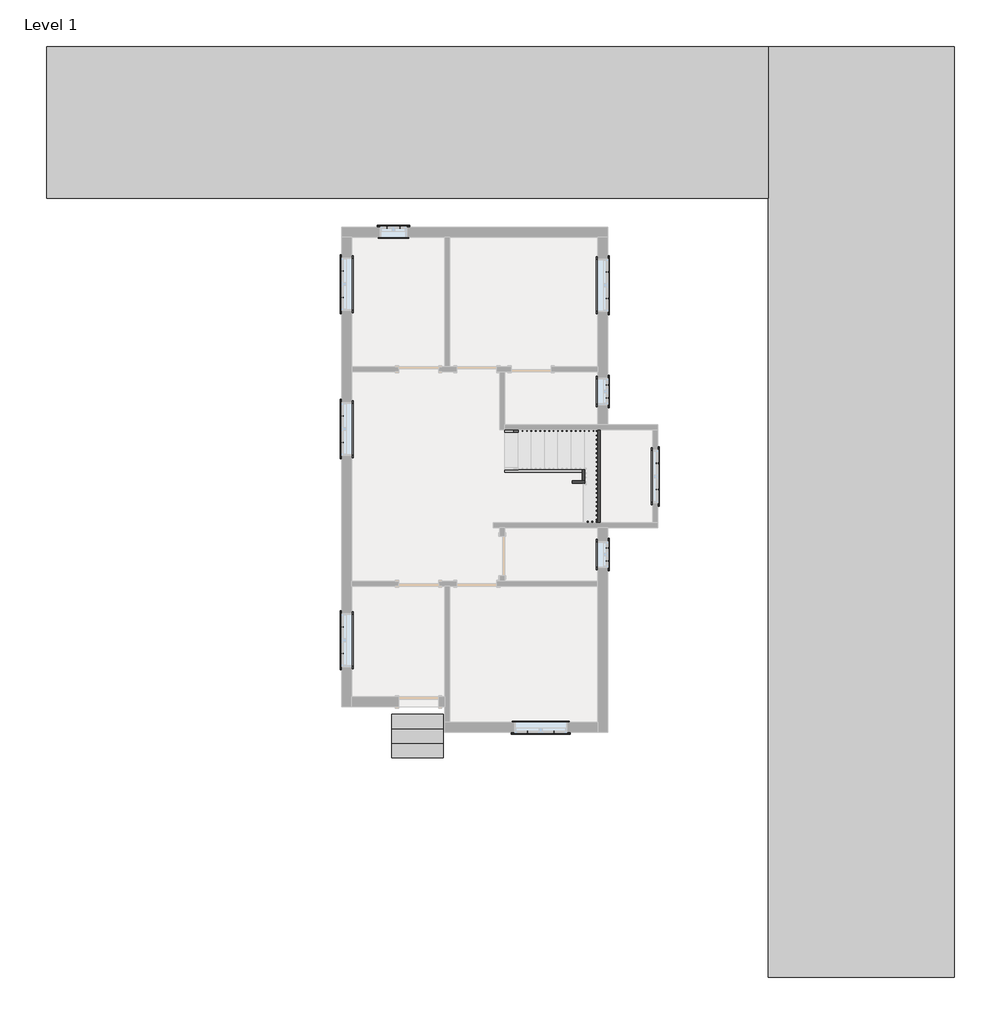
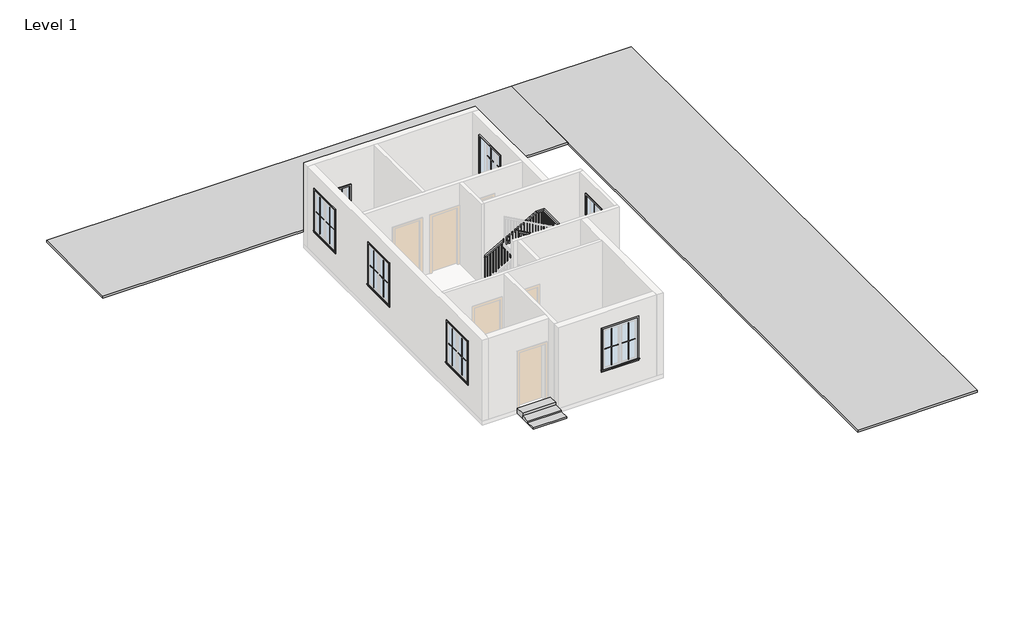
# One storey, part 2 of 2: 38 proxies, 4 members, 1 railing.
"""IFC4 building model written with IfcOpenShell, lengths in millimetres."""

from ifc_helpers import new_model, si_unit, frame, origin, place, context, project, spatial, polyline, outline, extrude, faceted_brep, transform, mapped, element, save
from components import generic_models_1_generic_models_1_85262742, generic_models_2_generic_models_2_51d3bdcd, muntin_pattern_2x2_muntin_pattern_2x2_6dad3731, muntin_pattern_2x2_muntin_pattern_2x2_a30a3345, muntin_pattern_2x2_muntin_pattern_2x2_53152e2c, muntin_pattern_2x2_muntin_pattern_2x2_e8f3e573, trim_window_exterior_flat_with_sill_92b9b949, trim_window_exterior_flat_with_sill_a665a915, trim_window_interior_flat_picture_frame_3bb882cf, trim_window_interior_flat_picture_frame_d485c387

model = new_model("IFC4")

# Units and contexts
model_context = context("Model", 3, world=origin())
ifc_project = project(units=[si_unit("LENGTHUNIT", "METRE", prefix="MILLI")], contexts=[model_context])

# Site, building, storey
site = spatial("IfcSite", under=ifc_project)
building = spatial("IfcBuilding", under=site)
storey = spatial("IfcBuildingStorey", under=building, Name="Level 1", Elevation=0.0)

# Proxies
placement = place(None, origin())
generic_models_1_generic_models_1_shape = generic_models_1_generic_models_1_85262742(model_context)
element("IfcBuildingElementProxy", 1, Name="Generic Models 1 : Generic Models 1", ObjectType="Generic Models 1 : Generic Models 1", at=placement, inside=storey, context=model_context, shape_type="MappedRepresentation", body=[
    mapped(generic_models_1_generic_models_1_shape, transform((0.0, 0.0, 0.0), x_axis=(1.0, 0.0, 0.0), y_axis=(0.0, 1.0, 0.0), z_axis=(0.0, 0.0, 1.0))),
])
generic_models_2_generic_models_2_shape = generic_models_2_generic_models_2_51d3bdcd(model_context)
element("IfcBuildingElementProxy", 2, Name="Generic Models 2 : Generic Models 2", ObjectType="Generic Models 2 : Generic Models 2", at=placement, inside=storey, context=model_context, shape_type="MappedRepresentation", body=[
    mapped(generic_models_2_generic_models_2_shape, transform((0.0, 0.0, 0.0), x_axis=(1.0, 0.0, 0.0), y_axis=(0.0, 1.0, 0.0), z_axis=(0.0, 0.0, 1.0))),
])
muntin_pattern_2x2_muntin_pattern_2x2_shape = muntin_pattern_2x2_muntin_pattern_2x2_6dad3731(model_context)
element("IfcBuildingElementProxy", 3, Name="Muntin Pattern_2x2 : Muntin Pattern_2x2", ObjectType="Muntin Pattern_2x2 : Muntin Pattern_2x2", at=placement, inside=storey, context=model_context, shape_type="MappedRepresentation", body=[
    mapped(muntin_pattern_2x2_muntin_pattern_2x2_shape, transform((1279.525, 12612.6875, 984.25), x_axis=(0.0, 1.0, 0.0), y_axis=(-1.0, 0.0, 0.0), z_axis=(0.0, 0.0, 1.0))),
])
element("IfcBuildingElementProxy", 4, Name="Muntin Pattern_2x2 : Muntin Pattern_2x2", ObjectType="Muntin Pattern_2x2 : Muntin Pattern_2x2", at=placement, inside=storey, context=model_context, shape_type="MappedRepresentation", body=[
    mapped(muntin_pattern_2x2_muntin_pattern_2x2_shape, transform((7356.475, 13193.7125, 984.25), x_axis=(0.0, -1.0, 0.0), y_axis=(1.0, 0.0, 0.0), z_axis=(0.0, 0.0, 1.0))),
])
element("IfcBuildingElementProxy", 5, Name="Muntin Pattern_2x2 : Muntin Pattern_2x2", ObjectType="Muntin Pattern_2x2 : Muntin Pattern_2x2", at=placement, inside=storey, context=model_context, shape_type="MappedRepresentation", body=[
    mapped(muntin_pattern_2x2_muntin_pattern_2x2_shape, transform((8499.475, 8812.2125, 984.25), x_axis=(0.0, -1.0, 0.0), y_axis=(1.0, 0.0, 0.0), z_axis=(0.0, 0.0, 1.0))),
])
element("IfcBuildingElementProxy", 6, Name="Muntin Pattern_2x2 : Muntin Pattern_2x2", ObjectType="Muntin Pattern_2x2 : Muntin Pattern_2x2", at=placement, inside=storey, context=model_context, shape_type="MappedRepresentation", body=[
    mapped(muntin_pattern_2x2_muntin_pattern_2x2_shape, transform((6132.5125, 2651.125, 984.25), x_axis=(-1.0, 0.0, 0.0), y_axis=(0.0, -1.0, 0.0), z_axis=(0.0, 0.0, 1.0))),
])
element("IfcBuildingElementProxy", 7, Name="Muntin Pattern_2x2 : Muntin Pattern_2x2", ObjectType="Muntin Pattern_2x2 : Muntin Pattern_2x2", at=placement, inside=storey, context=model_context, shape_type="MappedRepresentation", body=[
    mapped(muntin_pattern_2x2_muntin_pattern_2x2_shape, transform((1279.525, 4452.9375, 984.25), x_axis=(0.0, 1.0, 0.0), y_axis=(-1.0, 0.0, 0.0), z_axis=(0.0, 0.0, 1.0))),
])
element("IfcBuildingElementProxy", 8, Name="Muntin Pattern_2x2 : Muntin Pattern_2x2", ObjectType="Muntin Pattern_2x2 : Muntin Pattern_2x2", at=placement, inside=storey, context=model_context, shape_type="MappedRepresentation", body=[
    mapped(muntin_pattern_2x2_muntin_pattern_2x2_shape, transform((1279.525, 9291.6375, 984.25), x_axis=(0.0, 1.0, 0.0), y_axis=(-1.0, 0.0, 0.0), z_axis=(0.0, 0.0, 1.0))),
])
muntin_pattern_2x2_muntin_pattern_2x2_2_shape = muntin_pattern_2x2_muntin_pattern_2x2_a30a3345(model_context)
element("IfcBuildingElementProxy", 9, Name="Muntin Pattern_2x2 : Muntin Pattern_2x2", ObjectType="Muntin Pattern_2x2 : Muntin Pattern_2x2", at=placement, inside=storey, context=model_context, shape_type="MappedRepresentation", body=[
    mapped(muntin_pattern_2x2_muntin_pattern_2x2_2_shape, transform((1279.525, 13219.1125, 984.25), x_axis=(0.0, -1.0, 0.0), y_axis=(1.0, 0.0, 0.0), z_axis=(0.0, 0.0, 1.0))),
])
element("IfcBuildingElementProxy", 10, Name="Muntin Pattern_2x2 : Muntin Pattern_2x2", ObjectType="Muntin Pattern_2x2 : Muntin Pattern_2x2", at=placement, inside=storey, context=model_context, shape_type="MappedRepresentation", body=[
    mapped(muntin_pattern_2x2_muntin_pattern_2x2_2_shape, transform((7356.475, 12587.2875, 984.25), x_axis=(0.0, 1.0, 0.0), y_axis=(-1.0, 0.0, 0.0), z_axis=(0.0, 0.0, 1.0))),
])
element("IfcBuildingElementProxy", 11, Name="Muntin Pattern_2x2 : Muntin Pattern_2x2", ObjectType="Muntin Pattern_2x2 : Muntin Pattern_2x2", at=placement, inside=storey, context=model_context, shape_type="MappedRepresentation", body=[
    mapped(muntin_pattern_2x2_muntin_pattern_2x2_2_shape, transform((8499.475, 8205.7875, 984.25), x_axis=(0.0, 1.0, 0.0), y_axis=(-1.0, 0.0, 0.0), z_axis=(0.0, 0.0, 1.0))),
])
element("IfcBuildingElementProxy", 12, Name="Muntin Pattern_2x2 : Muntin Pattern_2x2", ObjectType="Muntin Pattern_2x2 : Muntin Pattern_2x2", at=placement, inside=storey, context=model_context, shape_type="MappedRepresentation", body=[
    mapped(muntin_pattern_2x2_muntin_pattern_2x2_2_shape, transform((5526.0875, 2651.125, 984.25), x_axis=(1.0, 0.0, 0.0), y_axis=(0.0, 1.0, 0.0), z_axis=(0.0, 0.0, 1.0))),
])
element("IfcBuildingElementProxy", 13, Name="Muntin Pattern_2x2 : Muntin Pattern_2x2", ObjectType="Muntin Pattern_2x2 : Muntin Pattern_2x2", at=placement, inside=storey, context=model_context, shape_type="MappedRepresentation", body=[
    mapped(muntin_pattern_2x2_muntin_pattern_2x2_2_shape, transform((1279.525, 5059.3625, 984.25), x_axis=(0.0, -1.0, 0.0), y_axis=(1.0, 0.0, 0.0), z_axis=(0.0, 0.0, 1.0))),
])
element("IfcBuildingElementProxy", 14, Name="Muntin Pattern_2x2 : Muntin Pattern_2x2", ObjectType="Muntin Pattern_2x2 : Muntin Pattern_2x2", at=placement, inside=storey, context=model_context, shape_type="MappedRepresentation", body=[
    mapped(muntin_pattern_2x2_muntin_pattern_2x2_2_shape, transform((1279.525, 9898.0625, 984.25), x_axis=(0.0, -1.0, 0.0), y_axis=(1.0, 0.0, 0.0), z_axis=(0.0, 0.0, 1.0))),
])
muntin_pattern_2x2_muntin_pattern_2x2_3_shape = muntin_pattern_2x2_muntin_pattern_2x2_53152e2c(model_context)
element("IfcBuildingElementProxy", 15, Name="Muntin Pattern_2x2 : Muntin Pattern_2x2", ObjectType="Muntin Pattern_2x2 : Muntin Pattern_2x2", at=placement, inside=storey, context=model_context, shape_type="MappedRepresentation", body=[
    mapped(muntin_pattern_2x2_muntin_pattern_2x2_3_shape, transform((2300.2875, 14214.475, 984.25), x_axis=(1.0, 0.0, 0.0), y_axis=(0.0, 1.0, 0.0), z_axis=(0.0, 0.0, 1.0))),
])
element("IfcBuildingElementProxy", 16, Name="Muntin Pattern_2x2 : Muntin Pattern_2x2", ObjectType="Muntin Pattern_2x2 : Muntin Pattern_2x2", at=placement, inside=storey, context=model_context, shape_type="MappedRepresentation", body=[
    mapped(muntin_pattern_2x2_muntin_pattern_2x2_3_shape, transform((7356.475, 10609.2625, 984.25), x_axis=(0.0, -1.0, 0.0), y_axis=(1.0, 0.0, 0.0), z_axis=(0.0, 0.0, 1.0))),
])
element("IfcBuildingElementProxy", 17, Name="Muntin Pattern_2x2 : Muntin Pattern_2x2", ObjectType="Muntin Pattern_2x2 : Muntin Pattern_2x2", at=placement, inside=storey, context=model_context, shape_type="MappedRepresentation", body=[
    mapped(muntin_pattern_2x2_muntin_pattern_2x2_3_shape, transform((7356.475, 6869.1125, 984.25), x_axis=(0.0, -1.0, 0.0), y_axis=(1.0, 0.0, 0.0), z_axis=(0.0, 0.0, 1.0))),
])
muntin_pattern_2x2_muntin_pattern_2x2_4_shape = muntin_pattern_2x2_muntin_pattern_2x2_e8f3e573(model_context)
element("IfcBuildingElementProxy", 18, Name="Muntin Pattern_2x2 : Muntin Pattern_2x2", ObjectType="Muntin Pattern_2x2 : Muntin Pattern_2x2", at=placement, inside=storey, context=model_context, shape_type="MappedRepresentation", body=[
    mapped(muntin_pattern_2x2_muntin_pattern_2x2_4_shape, transform((2601.9125, 14214.475, 984.25), x_axis=(-1.0, 0.0, 0.0), y_axis=(0.0, -1.0, 0.0), z_axis=(0.0, 0.0, 1.0))),
])
element("IfcBuildingElementProxy", 19, Name="Muntin Pattern_2x2 : Muntin Pattern_2x2", ObjectType="Muntin Pattern_2x2 : Muntin Pattern_2x2", at=placement, inside=storey, context=model_context, shape_type="MappedRepresentation", body=[
    mapped(muntin_pattern_2x2_muntin_pattern_2x2_4_shape, transform((7356.475, 10307.6375, 984.25), x_axis=(0.0, 1.0, 0.0), y_axis=(-1.0, 0.0, 0.0), z_axis=(0.0, 0.0, 1.0))),
])
element("IfcBuildingElementProxy", 20, Name="Muntin Pattern_2x2 : Muntin Pattern_2x2", ObjectType="Muntin Pattern_2x2 : Muntin Pattern_2x2", at=placement, inside=storey, context=model_context, shape_type="MappedRepresentation", body=[
    mapped(muntin_pattern_2x2_muntin_pattern_2x2_4_shape, transform((7356.475, 6567.4875, 984.25), x_axis=(0.0, 1.0, 0.0), y_axis=(-1.0, 0.0, 0.0), z_axis=(0.0, 0.0, 1.0))),
])
trim_window_exterior_flat_with_sill_shape = trim_window_exterior_flat_with_sill_92b9b949(model_context)
element("IfcBuildingElementProxy", 21, Name="Trim-Window-Exterior-Flat : with Sill", ObjectType="Trim-Window-Exterior-Flat : with Sill", at=placement, inside=storey, context=model_context, shape_type="MappedRepresentation", body=[
    mapped(trim_window_exterior_flat_with_sill_shape, transform((1270.0, 12915.9, 2438.4), x_axis=(0.0, -1.0, 0.0), y_axis=(0.0, 0.0, 1.0), z_axis=(-1.0, 0.0, 0.0))),
])
element("IfcBuildingElementProxy", 22, Name="Trim-Window-Exterior-Flat : with Sill", ObjectType="Trim-Window-Exterior-Flat : with Sill", at=placement, inside=storey, context=model_context, shape_type="MappedRepresentation", body=[
    mapped(trim_window_exterior_flat_with_sill_shape, transform((7366.0, 12890.5, 2438.4), x_axis=(0.0, 1.0, 0.0), y_axis=(0.0, 0.0, 1.0), z_axis=(1.0, 0.0, 0.0))),
])
element("IfcBuildingElementProxy", 23, Name="Trim-Window-Exterior-Flat : with Sill", ObjectType="Trim-Window-Exterior-Flat : with Sill", at=placement, inside=storey, context=model_context, shape_type="MappedRepresentation", body=[
    mapped(trim_window_exterior_flat_with_sill_shape, transform((8509.0, 8509.0, 2438.4), x_axis=(0.0, 1.0, 0.0), y_axis=(0.0, 0.0, 1.0), z_axis=(1.0, 0.0, 0.0))),
])
element("IfcBuildingElementProxy", 24, Name="Trim-Window-Exterior-Flat : with Sill", ObjectType="Trim-Window-Exterior-Flat : with Sill", at=placement, inside=storey, context=model_context, shape_type="MappedRepresentation", body=[
    mapped(trim_window_exterior_flat_with_sill_shape, transform((5829.3, 2641.6, 2438.4), x_axis=(1.0, 0.0, 0.0), y_axis=(0.0, 0.0, 1.0), z_axis=(0.0, -1.0, 0.0))),
])
element("IfcBuildingElementProxy", 25, Name="Trim-Window-Exterior-Flat : with Sill", ObjectType="Trim-Window-Exterior-Flat : with Sill", at=placement, inside=storey, context=model_context, shape_type="MappedRepresentation", body=[
    mapped(trim_window_exterior_flat_with_sill_shape, transform((1270.0, 4756.15, 2438.4), x_axis=(0.0, -1.0, 0.0), y_axis=(0.0, 0.0, 1.0), z_axis=(-1.0, 0.0, 0.0))),
])
element("IfcBuildingElementProxy", 26, Name="Trim-Window-Exterior-Flat : with Sill", ObjectType="Trim-Window-Exterior-Flat : with Sill", at=placement, inside=storey, context=model_context, shape_type="MappedRepresentation", body=[
    mapped(trim_window_exterior_flat_with_sill_shape, transform((1270.0, 9594.85, 2438.4), x_axis=(0.0, -1.0, 0.0), y_axis=(0.0, 0.0, 1.0), z_axis=(-1.0, 0.0, 0.0))),
])
trim_window_exterior_flat_with_sill_2_shape = trim_window_exterior_flat_with_sill_a665a915(model_context)
element("IfcBuildingElementProxy", 27, Name="Trim-Window-Exterior-Flat : with Sill", ObjectType="Trim-Window-Exterior-Flat : with Sill", at=placement, inside=storey, context=model_context, shape_type="MappedRepresentation", body=[
    mapped(trim_window_exterior_flat_with_sill_2_shape, transform((2451.1, 14224.0, 1828.8), x_axis=(-1.0, 0.0, 0.0), y_axis=(0.0, 0.0, 1.0), z_axis=(0.0, 1.0, 0.0))),
])
element("IfcBuildingElementProxy", 28, Name="Trim-Window-Exterior-Flat : with Sill", ObjectType="Trim-Window-Exterior-Flat : with Sill", at=placement, inside=storey, context=model_context, shape_type="MappedRepresentation", body=[
    mapped(trim_window_exterior_flat_with_sill_2_shape, transform((7366.0, 10458.45, 1828.8), x_axis=(0.0, 1.0, 0.0), y_axis=(0.0, 0.0, 1.0), z_axis=(1.0, 0.0, 0.0))),
])
element("IfcBuildingElementProxy", 29, Name="Trim-Window-Exterior-Flat : with Sill", ObjectType="Trim-Window-Exterior-Flat : with Sill", at=placement, inside=storey, context=model_context, shape_type="MappedRepresentation", body=[
    mapped(trim_window_exterior_flat_with_sill_2_shape, transform((7366.0, 6718.3, 1828.8), x_axis=(0.0, 1.0, 0.0), y_axis=(0.0, 0.0, 1.0), z_axis=(1.0, 0.0, 0.0))),
])
trim_window_interior_flat_picture_frame_shape = trim_window_interior_flat_picture_frame_3bb882cf(model_context)
element("IfcBuildingElementProxy", 30, Name="Trim-Window-Interior-Flat : Picture Frame", ObjectType="Trim-Window-Interior-Flat : Picture Frame", at=placement, inside=storey, context=model_context, shape_type="MappedRepresentation", body=[
    mapped(trim_window_interior_flat_picture_frame_shape, transform((1498.6, 12915.9, 2438.4), x_axis=(0.0, 1.0, 0.0), y_axis=(0.0, 0.0, 1.0), z_axis=(1.0, 0.0, 0.0))),
])
element("IfcBuildingElementProxy", 31, Name="Trim-Window-Interior-Flat : Picture Frame", ObjectType="Trim-Window-Interior-Flat : Picture Frame", at=placement, inside=storey, context=model_context, shape_type="MappedRepresentation", body=[
    mapped(trim_window_interior_flat_picture_frame_shape, transform((7137.4, 12890.5, 2438.4), x_axis=(0.0, -1.0, 0.0), y_axis=(0.0, 0.0, 1.0), z_axis=(-1.0, 0.0, 0.0))),
])
element("IfcBuildingElementProxy", 32, Name="Trim-Window-Interior-Flat : Picture Frame", ObjectType="Trim-Window-Interior-Flat : Picture Frame", at=placement, inside=storey, context=model_context, shape_type="MappedRepresentation", body=[
    mapped(trim_window_interior_flat_picture_frame_shape, transform((8394.7, 8509.0, 2438.4), x_axis=(0.0, -1.0, 0.0), y_axis=(0.0, 0.0, 1.0), z_axis=(-1.0, 0.0, 0.0))),
])
element("IfcBuildingElementProxy", 33, Name="Trim-Window-Interior-Flat : Picture Frame", ObjectType="Trim-Window-Interior-Flat : Picture Frame", at=placement, inside=storey, context=model_context, shape_type="MappedRepresentation", body=[
    mapped(trim_window_interior_flat_picture_frame_shape, transform((5829.3, 2870.2, 2438.4), x_axis=(-1.0, 0.0, 0.0), y_axis=(0.0, 0.0, 1.0), z_axis=(0.0, 1.0, 0.0))),
])
element("IfcBuildingElementProxy", 34, Name="Trim-Window-Interior-Flat : Picture Frame", ObjectType="Trim-Window-Interior-Flat : Picture Frame", at=placement, inside=storey, context=model_context, shape_type="MappedRepresentation", body=[
    mapped(trim_window_interior_flat_picture_frame_shape, transform((1498.6, 4756.15, 2438.4), x_axis=(0.0, 1.0, 0.0), y_axis=(0.0, 0.0, 1.0), z_axis=(1.0, 0.0, 0.0))),
])
element("IfcBuildingElementProxy", 35, Name="Trim-Window-Interior-Flat : Picture Frame", ObjectType="Trim-Window-Interior-Flat : Picture Frame", at=placement, inside=storey, context=model_context, shape_type="MappedRepresentation", body=[
    mapped(trim_window_interior_flat_picture_frame_shape, transform((1498.6, 9594.85, 2438.4), x_axis=(0.0, 1.0, 0.0), y_axis=(0.0, 0.0, 1.0), z_axis=(1.0, 0.0, 0.0))),
])
trim_window_interior_flat_picture_frame_2_shape = trim_window_interior_flat_picture_frame_d485c387(model_context)
element("IfcBuildingElementProxy", 36, Name="Trim-Window-Interior-Flat : Picture Frame", ObjectType="Trim-Window-Interior-Flat : Picture Frame", at=placement, inside=storey, context=model_context, shape_type="MappedRepresentation", body=[
    mapped(trim_window_interior_flat_picture_frame_2_shape, transform((2451.1, 13995.4, 1828.8), x_axis=(1.0, 0.0, 0.0), y_axis=(0.0, 0.0, 1.0), z_axis=(0.0, -1.0, 0.0))),
])
element("IfcBuildingElementProxy", 37, Name="Trim-Window-Interior-Flat : Picture Frame", ObjectType="Trim-Window-Interior-Flat : Picture Frame", at=placement, inside=storey, context=model_context, shape_type="MappedRepresentation", body=[
    mapped(trim_window_interior_flat_picture_frame_2_shape, transform((7137.4, 10458.45, 1828.8), x_axis=(0.0, -1.0, 0.0), y_axis=(0.0, 0.0, 1.0), z_axis=(-1.0, 0.0, 0.0))),
])
element("IfcBuildingElementProxy", 38, Name="Trim-Window-Interior-Flat : Picture Frame", ObjectType="Trim-Window-Interior-Flat : Picture Frame", at=placement, inside=storey, context=model_context, shape_type="MappedRepresentation", body=[
    mapped(trim_window_interior_flat_picture_frame_2_shape, transform((7137.4, 6718.3, 1828.8), x_axis=(0.0, -1.0, 0.0), y_axis=(0.0, 0.0, 1.0), z_axis=(-1.0, 0.0, 0.0))),
])

# Members
element("IfcMember", 39, ObjectType="Stringer - 2\" Width", at=placement, inside=storey, context=model_context, shape_type="SweptSolid", body=[
    extrude(outline(polyline([(7137.4, 9575.8), (7188.2, 9575.8), (7188.2, 7442.2), (7137.4, 7442.2), (7137.4, 9575.8)])), frame((0.0, 0.0, 956.7333333), z_axis=(0.0, 0.0, 1.0), x_axis=(1.0, 0.0, 0.0)), (0.0, 0.0, 1.0), 304.8),
])
element("IfcMember", 40, ObjectType="Stringer - 2\" Width", at=placement, inside=storey, context=model_context, shape_type="SweptSolid", body=[
    extrude(outline(polyline([(207.5983948, 5003.8), (0.0, 5003.8), (0.0, 5257.7445028), (846.6974984, 6781.8), (1195.3761726, 6781.8), (207.5983948, 5003.8)])), frame((0.0, 8610.6, 0.0), z_axis=(0.0, 1.0, 0.0), x_axis=(0.0, 0.0, 1.0)), (0.0, 0.0, 1.0), 50.8),
])
element("IfcMember", 41, ObjectType="Stringer - 2\" Width", at=placement, inside=storey, context=model_context, shape_type="SweptSolid", body=[
    extrude(outline(polyline([(6781.8, 8661.4), (6832.6, 8661.4), (6832.6, 8407.4), (6781.8, 8407.4), (6781.8, 8661.4)])), frame((0.0, 0.0, 956.7333333), z_axis=(0.0, 0.0, 1.0), x_axis=(1.0, 0.0, 0.0)), (0.0, 0.0, 1.0), 304.8),
])
element("IfcMember", 42, ObjectType="Stringer - 2\" Width", at=placement, inside=storey, context=model_context, shape_type="SweptSolid", body=[
    extrude(outline(polyline([(1044.253054, 6832.6), (1392.9317281, 6832.6), (2408.9317281, 5003.8), (2060.253054, 5003.8), (1044.253054, 6832.6)])), frame((0.0, 8356.6, 0.0), z_axis=(0.0, 1.0, 0.0), x_axis=(0.0, 0.0, 1.0)), (0.0, 0.0, 1.0), 50.8),
])

# Railing
element("IfcRailing", 43, ObjectType="Handrail - Rectangular", at=placement, inside=storey, context=model_context, shape_type="SolidModel", body=[
    faceted_brep([(5003.8, 9575.8, 1083.7333333), (5003.8, 9575.8, 1025.620221), (5003.8, 9525.0, 1025.620221), (5003.8, 9525.0, 1083.7333333), (6832.6, 9575.8, 2099.7333333), (6845.7636022, 9575.8, 2048.9333333), (6845.7636022, 9525.0, 2048.9333333), (6832.6, 9525.0, 2099.7333333), (7137.4, 9575.8, 2099.7333333), (7137.4, 9575.8, 2048.9333333), (7086.6, 9525.0, 2048.9333333), (7086.6, 9525.0, 2099.7333333), (7137.4, 7569.2, 2099.7333333), (7137.4, 7518.4, 2048.9333333), (7086.6, 7518.4, 2048.9333333), (7086.6, 7569.2, 2099.7333333), (7137.4, 7569.2, 2170.2888889), (7137.4, 7518.4, 2119.4888889), (7086.6, 7518.4, 2119.4888889), (7086.6, 7569.2, 2170.2888889), (7137.4, 7442.2, 2170.2888889), (7137.4, 7442.2, 2119.4888889), (7086.6, 7493.0, 2119.4888889), (7086.6, 7493.0, 2170.2888889), (7010.4, 7442.2, 2170.2888889), (6997.2363978, 7442.2, 2119.4888889), (6997.2363978, 7493.0, 2119.4888889), (7010.4, 7493.0, 2170.2888889), (5003.8, 7442.2, 3285.0666667), (5003.8, 7493.0, 3285.0666667), (5003.8, 7493.0, 3226.9535543), (5003.8, 7442.2, 3226.9535543)], [[[0, 1, 2, 3]], [[1, 0, 4, 5]], [[2, 1, 5, 6]], [[3, 2, 6, 7]], [[0, 3, 7, 4]], [[5, 4, 8, 9]], [[6, 5, 9, 10]], [[7, 6, 10, 11]], [[4, 7, 11, 8]], [[9, 8, 12, 13]], [[10, 9, 13, 14]], [[11, 10, 14, 15]], [[8, 11, 15, 12]], [[13, 12, 16, 17]], [[14, 13, 17, 18]], [[15, 14, 18, 19]], [[12, 15, 19, 16]], [[17, 16, 20, 21]], [[18, 17, 21, 22]], [[19, 18, 22, 23]], [[16, 19, 23, 20]], [[21, 20, 24, 25]], [[22, 21, 25, 26]], [[23, 22, 26, 27]], [[20, 23, 27, 24]], [[28, 29, 30, 31]], [[25, 24, 28, 31]], [[26, 25, 31, 30]], [[27, 26, 30, 29]], [[24, 27, 29, 28]]]),
    extrude(outline(polyline([(3189.9118876, 5070.475), (2201.3333333, 5070.475), (2201.3333333, 5089.525), (3179.3285543, 5089.525), (3189.9118876, 5070.475)])), frame((0.0, 7458.075, 0.0), z_axis=(0.0, 1.0, 0.0), x_axis=(0.0, 0.0, 1.0)), (0.0, 0.0, 1.0), 19.05),
    extrude(outline(polyline([(3133.4674432, 5172.075), (2201.3333333, 5172.075), (2201.3333333, 5191.125), (3122.8841099, 5191.125), (3133.4674432, 5172.075)])), frame((0.0, 7458.075, 0.0), z_axis=(0.0, 1.0, 0.0), x_axis=(0.0, 0.0, 1.0)), (0.0, 0.0, 1.0), 19.05),
    extrude(outline(polyline([(3077.0229988, 5273.675), (2201.3333333, 5273.675), (2201.3333333, 5292.725), (3066.4396654, 5292.725), (3077.0229988, 5273.675)])), frame((0.0, 7458.075, 0.0), z_axis=(0.0, 1.0, 0.0), x_axis=(0.0, 0.0, 1.0)), (0.0, 0.0, 1.0), 19.05),
    extrude(outline(polyline([(3020.5785543, 5375.275), (2032.0, 5375.275), (2032.0, 5394.325), (3009.995221, 5394.325), (3020.5785543, 5375.275)])), frame((0.0, 7458.075, 0.0), z_axis=(0.0, 1.0, 0.0), x_axis=(0.0, 0.0, 1.0)), (0.0, 0.0, 1.0), 19.05),
    extrude(outline(polyline([(2964.1341099, 5476.875), (2032.0, 5476.875), (2032.0, 5495.925), (2953.5507765, 5495.925), (2964.1341099, 5476.875)])), frame((0.0, 7458.075, 0.0), z_axis=(0.0, 1.0, 0.0), x_axis=(0.0, 0.0, 1.0)), (0.0, 0.0, 1.0), 19.05),
    extrude(outline(polyline([(2907.6896654, 5578.475), (2032.0, 5578.475), (2032.0, 5597.525), (2897.1063321, 5597.525), (2907.6896654, 5578.475)])), frame((0.0, 7458.075, 0.0), z_axis=(0.0, 1.0, 0.0), x_axis=(0.0, 0.0, 1.0)), (0.0, 0.0, 1.0), 19.05),
    extrude(outline(polyline([(2851.245221, 5680.075), (1862.6666667, 5680.075), (1862.6666667, 5699.125), (2840.6618876, 5699.125), (2851.245221, 5680.075)])), frame((0.0, 7458.075, 0.0), z_axis=(0.0, 1.0, 0.0), x_axis=(0.0, 0.0, 1.0)), (0.0, 0.0, 1.0), 19.05),
    extrude(outline(polyline([(2794.8007765, 5781.675), (1862.6666667, 5781.675), (1862.6666667, 5800.725), (2784.2174432, 5800.725), (2794.8007765, 5781.675)])), frame((0.0, 7458.075, 0.0), z_axis=(0.0, 1.0, 0.0), x_axis=(0.0, 0.0, 1.0)), (0.0, 0.0, 1.0), 19.05),
    extrude(outline(polyline([(2738.3563321, 5883.275), (1862.6666667, 5883.275), (1862.6666667, 5902.325), (2727.7729988, 5902.325), (2738.3563321, 5883.275)])), frame((0.0, 7458.075, 0.0), z_axis=(0.0, 1.0, 0.0), x_axis=(0.0, 0.0, 1.0)), (0.0, 0.0, 1.0), 19.05),
    extrude(outline(polyline([(2681.9118876, 5984.875), (1693.3333333, 5984.875), (1693.3333333, 6003.925), (2671.3285543, 6003.925), (2681.9118876, 5984.875)])), frame((0.0, 7458.075, 0.0), z_axis=(0.0, 1.0, 0.0), x_axis=(0.0, 0.0, 1.0)), (0.0, 0.0, 1.0), 19.05),
    extrude(outline(polyline([(2625.4674432, 6086.475), (1693.3333333, 6086.475), (1693.3333333, 6105.525), (2614.8841099, 6105.525), (2625.4674432, 6086.475)])), frame((0.0, 7458.075, 0.0), z_axis=(0.0, 1.0, 0.0), x_axis=(0.0, 0.0, 1.0)), (0.0, 0.0, 1.0), 19.05),
    extrude(outline(polyline([(2569.0229988, 6188.075), (1693.3333333, 6188.075), (1693.3333333, 6207.125), (2558.4396654, 6207.125), (2569.0229988, 6188.075)])), frame((0.0, 7458.075, 0.0), z_axis=(0.0, 1.0, 0.0), x_axis=(0.0, 0.0, 1.0)), (0.0, 0.0, 1.0), 19.05),
    extrude(outline(polyline([(2512.5785543, 6289.675), (1524.0, 6289.675), (1524.0, 6308.725), (2501.995221, 6308.725), (2512.5785543, 6289.675)])), frame((0.0, 7458.075, 0.0), z_axis=(0.0, 1.0, 0.0), x_axis=(0.0, 0.0, 1.0)), (0.0, 0.0, 1.0), 19.05),
    extrude(outline(polyline([(2456.1341099, 6391.275), (1524.0, 6391.275), (1524.0, 6410.325), (2445.5507765, 6410.325), (2456.1341099, 6391.275)])), frame((0.0, 7458.075, 0.0), z_axis=(0.0, 1.0, 0.0), x_axis=(0.0, 0.0, 1.0)), (0.0, 0.0, 1.0), 19.05),
    extrude(outline(polyline([(2399.6896654, 6492.875), (1524.0, 6492.875), (1524.0, 6511.925), (2389.1063321, 6511.925), (2399.6896654, 6492.875)])), frame((0.0, 7458.075, 0.0), z_axis=(0.0, 1.0, 0.0), x_axis=(0.0, 0.0, 1.0)), (0.0, 0.0, 1.0), 19.05),
    extrude(outline(polyline([(2343.245221, 6594.475), (1354.6666667, 6594.475), (1354.6666667, 6613.525), (2332.6618876, 6613.525), (2343.245221, 6594.475)])), frame((0.0, 7458.075, 0.0), z_axis=(0.0, 1.0, 0.0), x_axis=(0.0, 0.0, 1.0)), (0.0, 0.0, 1.0), 19.05),
    extrude(outline(polyline([(2286.8007765, 6696.075), (1354.6666667, 6696.075), (1354.6666667, 6715.125), (2276.2174432, 6715.125), (2286.8007765, 6696.075)])), frame((0.0, 7458.075, 0.0), z_axis=(0.0, 1.0, 0.0), x_axis=(0.0, 0.0, 1.0)), (0.0, 0.0, 1.0), 19.05),
    extrude(outline(polyline([(2230.3563321, 6797.675), (1354.6666667, 6797.675), (1354.6666667, 6816.725), (2219.7729988, 6816.725), (2230.3563321, 6797.675)])), frame((0.0, 7458.075, 0.0), z_axis=(0.0, 1.0, 0.0), x_axis=(0.0, 0.0, 1.0)), (0.0, 0.0, 1.0), 19.05),
    extrude(outline(polyline([(2173.9118876, 6899.275), (1185.3333333, 6899.275), (1185.3333333, 6918.325), (2163.3285543, 6918.325), (2173.9118876, 6899.275)])), frame((0.0, 7458.075, 0.0), z_axis=(0.0, 1.0, 0.0), x_axis=(0.0, 0.0, 1.0)), (0.0, 0.0, 1.0), 19.05),
    extrude(outline(polyline([(2117.4674432, 7000.875), (1185.3333333, 7000.875), (1185.3333333, 7019.925), (2106.8841099, 7019.925), (2117.4674432, 7000.875)])), frame((0.0, 7458.075, 0.0), z_axis=(0.0, 1.0, 0.0), x_axis=(0.0, 0.0, 1.0)), (0.0, 0.0, 1.0), 19.05),
    extrude(outline(polyline([(7121.525, 7527.925), (7121.525, 7508.875), (7102.475, 7508.875), (7102.475, 7527.925), (7121.525, 7527.925)])), frame((0.0, 0.0, 1185.3333333), z_axis=(0.0, 0.0, 1.0), x_axis=(1.0, 0.0, 0.0)), (0.0, 0.0, 1.0), 934.1555556),
    extrude(outline(polyline([(7121.525, 7629.525), (7121.525, 7610.475), (7102.475, 7610.475), (7102.475, 7629.525), (7121.525, 7629.525)])), frame((0.0, 0.0, 1185.3333333), z_axis=(0.0, 0.0, 1.0), x_axis=(1.0, 0.0, 0.0)), (0.0, 0.0, 1.0), 863.6),
    extrude(outline(polyline([(7121.525, 7731.125), (7121.525, 7712.075), (7102.475, 7712.075), (7102.475, 7731.125), (7121.525, 7731.125)])), frame((0.0, 0.0, 1185.3333333), z_axis=(0.0, 0.0, 1.0), x_axis=(1.0, 0.0, 0.0)), (0.0, 0.0, 1.0), 863.6),
    extrude(outline(polyline([(7121.525, 7832.725), (7121.525, 7813.675), (7102.475, 7813.675), (7102.475, 7832.725), (7121.525, 7832.725)])), frame((0.0, 0.0, 1185.3333333), z_axis=(0.0, 0.0, 1.0), x_axis=(1.0, 0.0, 0.0)), (0.0, 0.0, 1.0), 863.6),
    extrude(outline(polyline([(7121.525, 7934.325), (7121.525, 7915.275), (7102.475, 7915.275), (7102.475, 7934.325), (7121.525, 7934.325)])), frame((0.0, 0.0, 1185.3333333), z_axis=(0.0, 0.0, 1.0), x_axis=(1.0, 0.0, 0.0)), (0.0, 0.0, 1.0), 863.6),
    extrude(outline(polyline([(7121.525, 8035.925), (7121.525, 8016.875), (7102.475, 8016.875), (7102.475, 8035.925), (7121.525, 8035.925)])), frame((0.0, 0.0, 1185.3333333), z_axis=(0.0, 0.0, 1.0), x_axis=(1.0, 0.0, 0.0)), (0.0, 0.0, 1.0), 863.6),
    extrude(outline(polyline([(7121.525, 8137.525), (7121.525, 8118.475), (7102.475, 8118.475), (7102.475, 8137.525), (7121.525, 8137.525)])), frame((0.0, 0.0, 1185.3333333), z_axis=(0.0, 0.0, 1.0), x_axis=(1.0, 0.0, 0.0)), (0.0, 0.0, 1.0), 863.6),
    extrude(outline(polyline([(7121.525, 8239.125), (7121.525, 8220.075), (7102.475, 8220.075), (7102.475, 8239.125), (7121.525, 8239.125)])), frame((0.0, 0.0, 1185.3333333), z_axis=(0.0, 0.0, 1.0), x_axis=(1.0, 0.0, 0.0)), (0.0, 0.0, 1.0), 863.6),
    extrude(outline(polyline([(7121.525, 8340.725), (7121.525, 8321.675), (7102.475, 8321.675), (7102.475, 8340.725), (7121.525, 8340.725)])), frame((0.0, 0.0, 1185.3333333), z_axis=(0.0, 0.0, 1.0), x_axis=(1.0, 0.0, 0.0)), (0.0, 0.0, 1.0), 863.6),
    extrude(outline(polyline([(7121.525, 8442.325), (7121.525, 8423.275), (7102.475, 8423.275), (7102.475, 8442.325), (7121.525, 8442.325)])), frame((0.0, 0.0, 1185.3333333), z_axis=(0.0, 0.0, 1.0), x_axis=(1.0, 0.0, 0.0)), (0.0, 0.0, 1.0), 863.6),
    extrude(outline(polyline([(7121.525, 8543.925), (7121.525, 8524.875), (7102.475, 8524.875), (7102.475, 8543.925), (7121.525, 8543.925)])), frame((0.0, 0.0, 1185.3333333), z_axis=(0.0, 0.0, 1.0), x_axis=(1.0, 0.0, 0.0)), (0.0, 0.0, 1.0), 863.6),
    extrude(outline(polyline([(7121.525, 8645.525), (7121.525, 8626.475), (7102.475, 8626.475), (7102.475, 8645.525), (7121.525, 8645.525)])), frame((0.0, 0.0, 1185.3333333), z_axis=(0.0, 0.0, 1.0), x_axis=(1.0, 0.0, 0.0)), (0.0, 0.0, 1.0), 863.6),
    extrude(outline(polyline([(7121.525, 8747.125), (7121.525, 8728.075), (7102.475, 8728.075), (7102.475, 8747.125), (7121.525, 8747.125)])), frame((0.0, 0.0, 1185.3333333), z_axis=(0.0, 0.0, 1.0), x_axis=(1.0, 0.0, 0.0)), (0.0, 0.0, 1.0), 863.6),
    extrude(outline(polyline([(7121.525, 8848.725), (7121.525, 8829.675), (7102.475, 8829.675), (7102.475, 8848.725), (7121.525, 8848.725)])), frame((0.0, 0.0, 1185.3333333), z_axis=(0.0, 0.0, 1.0), x_axis=(1.0, 0.0, 0.0)), (0.0, 0.0, 1.0), 863.6),
    extrude(outline(polyline([(7121.525, 8950.325), (7121.525, 8931.275), (7102.475, 8931.275), (7102.475, 8950.325), (7121.525, 8950.325)])), frame((0.0, 0.0, 1185.3333333), z_axis=(0.0, 0.0, 1.0), x_axis=(1.0, 0.0, 0.0)), (0.0, 0.0, 1.0), 863.6),
    extrude(outline(polyline([(7121.525, 9051.925), (7121.525, 9032.875), (7102.475, 9032.875), (7102.475, 9051.925), (7121.525, 9051.925)])), frame((0.0, 0.0, 1185.3333333), z_axis=(0.0, 0.0, 1.0), x_axis=(1.0, 0.0, 0.0)), (0.0, 0.0, 1.0), 863.6),
    extrude(outline(polyline([(7121.525, 9153.525), (7121.525, 9134.475), (7102.475, 9134.475), (7102.475, 9153.525), (7121.525, 9153.525)])), frame((0.0, 0.0, 1185.3333333), z_axis=(0.0, 0.0, 1.0), x_axis=(1.0, 0.0, 0.0)), (0.0, 0.0, 1.0), 863.6),
    extrude(outline(polyline([(7121.525, 9255.125), (7121.525, 9236.075), (7102.475, 9236.075), (7102.475, 9255.125), (7121.525, 9255.125)])), frame((0.0, 0.0, 1185.3333333), z_axis=(0.0, 0.0, 1.0), x_axis=(1.0, 0.0, 0.0)), (0.0, 0.0, 1.0), 863.6),
    extrude(outline(polyline([(7121.525, 9356.725), (7121.525, 9337.675), (7102.475, 9337.675), (7102.475, 9356.725), (7121.525, 9356.725)])), frame((0.0, 0.0, 1185.3333333), z_axis=(0.0, 0.0, 1.0), x_axis=(1.0, 0.0, 0.0)), (0.0, 0.0, 1.0), 863.6),
    extrude(outline(polyline([(7121.525, 9458.325), (7121.525, 9439.275), (7102.475, 9439.275), (7102.475, 9458.325), (7121.525, 9458.325)])), frame((0.0, 0.0, 1185.3333333), z_axis=(0.0, 0.0, 1.0), x_axis=(1.0, 0.0, 0.0)), (0.0, 0.0, 1.0), 863.6),
    extrude(outline(polyline([(7026.275, 9559.925), (7045.325, 9559.925), (7045.325, 9540.875), (7026.275, 9540.875), (7026.275, 9559.925)])), frame((0.0, 0.0, 1185.3333333), z_axis=(0.0, 0.0, 1.0), x_axis=(1.0, 0.0, 0.0)), (0.0, 0.0, 1.0), 863.6),
    extrude(outline(polyline([(6924.675, 9559.925), (6943.725, 9559.925), (6943.725, 9540.875), (6924.675, 9540.875), (6924.675, 9559.925)])), frame((0.0, 0.0, 1185.3333333), z_axis=(0.0, 0.0, 1.0), x_axis=(1.0, 0.0, 0.0)), (0.0, 0.0, 1.0), 863.6),
    extrude(outline(polyline([(2036.3285543, 6823.075), (1185.3333333, 6823.075), (1185.3333333, 6842.125), (2046.9118876, 6842.125), (2036.3285543, 6823.075)])), frame((0.0, 9540.875, 0.0), z_axis=(0.0, 1.0, 0.0), x_axis=(0.0, 0.0, 1.0)), (0.0, 0.0, 1.0), 19.05),
    extrude(outline(polyline([(1979.8841099, 6721.475), (1016.0, 6721.475), (1016.0, 6740.525), (1990.4674432, 6740.525), (1979.8841099, 6721.475)])), frame((0.0, 9540.875, 0.0), z_axis=(0.0, 1.0, 0.0), x_axis=(0.0, 0.0, 1.0)), (0.0, 0.0, 1.0), 19.05),
    extrude(outline(polyline([(1923.4396654, 6619.875), (1016.0, 6619.875), (1016.0, 6638.925), (1934.0229988, 6638.925), (1923.4396654, 6619.875)])), frame((0.0, 9540.875, 0.0), z_axis=(0.0, 1.0, 0.0), x_axis=(0.0, 0.0, 1.0)), (0.0, 0.0, 1.0), 19.05),
    extrude(outline(polyline([(1866.995221, 6518.275), (1016.0, 6518.275), (1016.0, 6537.325), (1877.5785543, 6537.325), (1866.995221, 6518.275)])), frame((0.0, 9540.875, 0.0), z_axis=(0.0, 1.0, 0.0), x_axis=(0.0, 0.0, 1.0)), (0.0, 0.0, 1.0), 19.05),
    extrude(outline(polyline([(1810.5507765, 6416.675), (846.6666667, 6416.675), (846.6666667, 6435.725), (1821.1341099, 6435.725), (1810.5507765, 6416.675)])), frame((0.0, 9540.875, 0.0), z_axis=(0.0, 1.0, 0.0), x_axis=(0.0, 0.0, 1.0)), (0.0, 0.0, 1.0), 19.05),
    extrude(outline(polyline([(1754.1063321, 6315.075), (846.6666667, 6315.075), (846.6666667, 6334.125), (1764.6896654, 6334.125), (1754.1063321, 6315.075)])), frame((0.0, 9540.875, 0.0), z_axis=(0.0, 1.0, 0.0), x_axis=(0.0, 0.0, 1.0)), (0.0, 0.0, 1.0), 19.05),
    extrude(outline(polyline([(1697.6618876, 6213.475), (846.6666667, 6213.475), (846.6666667, 6232.525), (1708.245221, 6232.525), (1697.6618876, 6213.475)])), frame((0.0, 9540.875, 0.0), z_axis=(0.0, 1.0, 0.0), x_axis=(0.0, 0.0, 1.0)), (0.0, 0.0, 1.0), 19.05),
    extrude(outline(polyline([(1641.2174432, 6111.875), (677.3333333, 6111.875), (677.3333333, 6130.925), (1651.8007765, 6130.925), (1641.2174432, 6111.875)])), frame((0.0, 9540.875, 0.0), z_axis=(0.0, 1.0, 0.0), x_axis=(0.0, 0.0, 1.0)), (0.0, 0.0, 1.0), 19.05),
    extrude(outline(polyline([(1584.7729988, 6010.275), (677.3333333, 6010.275), (677.3333333, 6029.325), (1595.3563321, 6029.325), (1584.7729988, 6010.275)])), frame((0.0, 9540.875, 0.0), z_axis=(0.0, 1.0, 0.0), x_axis=(0.0, 0.0, 1.0)), (0.0, 0.0, 1.0), 19.05),
    extrude(outline(polyline([(1528.3285543, 5908.675), (677.3333333, 5908.675), (677.3333333, 5927.725), (1538.9118876, 5927.725), (1528.3285543, 5908.675)])), frame((0.0, 9540.875, 0.0), z_axis=(0.0, 1.0, 0.0), x_axis=(0.0, 0.0, 1.0)), (0.0, 0.0, 1.0), 19.05),
    extrude(outline(polyline([(1471.8841099, 5807.075), (508.0, 5807.075), (508.0, 5826.125), (1482.4674432, 5826.125), (1471.8841099, 5807.075)])), frame((0.0, 9540.875, 0.0), z_axis=(0.0, 1.0, 0.0), x_axis=(0.0, 0.0, 1.0)), (0.0, 0.0, 1.0), 19.05),
    extrude(outline(polyline([(1415.4396654, 5705.475), (508.0, 5705.475), (508.0, 5724.525), (1426.0229988, 5724.525), (1415.4396654, 5705.475)])), frame((0.0, 9540.875, 0.0), z_axis=(0.0, 1.0, 0.0), x_axis=(0.0, 0.0, 1.0)), (0.0, 0.0, 1.0), 19.05),
    extrude(outline(polyline([(1358.995221, 5603.875), (508.0, 5603.875), (508.0, 5622.925), (1369.5785543, 5622.925), (1358.995221, 5603.875)])), frame((0.0, 9540.875, 0.0), z_axis=(0.0, 1.0, 0.0), x_axis=(0.0, 0.0, 1.0)), (0.0, 0.0, 1.0), 19.05),
    extrude(outline(polyline([(1302.5507765, 5502.275), (338.6666667, 5502.275), (338.6666667, 5521.325), (1313.1341099, 5521.325), (1302.5507765, 5502.275)])), frame((0.0, 9540.875, 0.0), z_axis=(0.0, 1.0, 0.0), x_axis=(0.0, 0.0, 1.0)), (0.0, 0.0, 1.0), 19.05),
    extrude(outline(polyline([(1246.1063321, 5400.675), (338.6666667, 5400.675), (338.6666667, 5419.725), (1256.6896654, 5419.725), (1246.1063321, 5400.675)])), frame((0.0, 9540.875, 0.0), z_axis=(0.0, 1.0, 0.0), x_axis=(0.0, 0.0, 1.0)), (0.0, 0.0, 1.0), 19.05),
    extrude(outline(polyline([(1189.6618876, 5299.075), (338.6666667, 5299.075), (338.6666667, 5318.125), (1200.245221, 5318.125), (1189.6618876, 5299.075)])), frame((0.0, 9540.875, 0.0), z_axis=(0.0, 1.0, 0.0), x_axis=(0.0, 0.0, 1.0)), (0.0, 0.0, 1.0), 19.05),
    extrude(outline(polyline([(1133.2174432, 5197.475), (169.3333333, 5197.475), (169.3333333, 5216.525), (1143.8007765, 5216.525), (1133.2174432, 5197.475)])), frame((0.0, 9540.875, 0.0), z_axis=(0.0, 1.0, 0.0), x_axis=(0.0, 0.0, 1.0)), (0.0, 0.0, 1.0), 19.05),
    extrude(outline(polyline([(1076.7729988, 5095.875), (169.3333333, 5095.875), (169.3333333, 5114.925), (1087.3563321, 5114.925), (1076.7729988, 5095.875)])), frame((0.0, 9540.875, 0.0), z_axis=(0.0, 1.0, 0.0), x_axis=(0.0, 0.0, 1.0)), (0.0, 0.0, 1.0), 19.05),
    extrude(outline(polyline([(7121.525, 7477.125), (7121.525, 7458.075), (7102.475, 7458.075), (7102.475, 7477.125), (7121.525, 7477.125)])), frame((0.0, 0.0, 1185.3333333), z_axis=(0.0, 0.0, 1.0), x_axis=(1.0, 0.0, 0.0)), (0.0, 0.0, 1.0), 934.1555556),
    extrude(outline(polyline([(7102.475, 9559.925), (7121.525, 9559.925), (7121.525, 9540.875), (7102.475, 9540.875), (7102.475, 9559.925)])), frame((0.0, 0.0, 1185.3333333), z_axis=(0.0, 0.0, 1.0), x_axis=(1.0, 0.0, 0.0)), (0.0, 0.0, 1.0), 863.6),
    extrude(outline(polyline([(3226.9535543, 5003.8), (2201.3333333, 5003.8), (2201.3333333, 5022.85), (3216.370221, 5022.85), (3226.9535543, 5003.8)])), frame((0.0, 7458.075, 0.0), z_axis=(0.0, 1.0, 0.0), x_axis=(0.0, 0.0, 1.0)), (0.0, 0.0, 1.0), 19.05),
    extrude(outline(polyline([(1025.620221, 5003.8), (169.3333333, 5003.8), (169.3333333, 5022.85), (1036.2035543, 5022.85), (1025.620221, 5003.8)])), frame((0.0, 9540.875, 0.0), z_axis=(0.0, 1.0, 0.0), x_axis=(0.0, 0.0, 1.0)), (0.0, 0.0, 1.0), 19.05),
])

save(model, "model.ifc")

# Revit data of these elements
# Type "Muntin Pattern_2x2 : Muntin Pattern_2x2"
#   Width [instance default] = 4' - 0"
#   Thickness = 0' - 0 1/2"
#   Height [instance default] = 4' - 0"
#   Distance = 0' - 0 3/4"
#   Interior Material [instance default] = none
#   Exterior Material [instance default] = none
#   Default Elevation = 0
# Type "Trim-Window-Exterior-Flat : with Sill"
#   Trim Width = 0' - 2 1/4"
#   Trim Thickness_Picture Frame = 0' - 1 1/4"
#   Trim Thickness_with Sill = 0' - 0 3/4"
#   Sill Thickness = 0' - 1 1/4"
#   Opening Width [instance default] = 2' - 0"
#   Opening Height [instance default] = 3' - 0"
#   Default Elevation = 4' - 0"
#   Sill = yes
#   Picture Frame = no
#   Trim Material [instance default] = none
# Type "Trim-Window-Interior-Flat : Picture Frame"
#   Trim Thickness_Picture Frame = 0' - 1 1/4"
#   Trim Width = 0' - 2 1/4"
#   Trim Thickness_with Sill = 0' - 0 3/4"
#   Sill Thickness = 0' - 1 1/4"
#   Opening Width [instance default] = 2' - 0"
#   Opening Height [instance default] = 3' - 0"
#   Default Elevation = 4' - 0"
#   Sill = no
#   Picture Frame = yes
#   Trim Material [instance default] = none
# Type "Handrail - Rectangular"
#   Assembly Code = "C2010400"
#   built-in parameter 1008612 = 0.0416667 (stored number, unit not read)
#   built-in parameter 1008611 = 0.0416667 (stored number, unit not read)
#   built-in parameter 1008609 = 0.333333 (stored number, unit not read)
#   built-in parameter 1008604 = 0.166667 (stored number, unit not read)
#   built-in parameter 1008603 = 0.166667 (stored number, unit not read)
#   Railing Height = 3' - 0"
#   built-in parameter 1008630 = 2
#   built-in parameter 1008610 = 2
#   built-in parameter 1008618 = Baluster - Square : 3/4"
# Element 1 (IfcBuildingElementProxy, "Generic Models 1 : Generic Models 1")
#   Phase Created = New Construction
# Element 2 (IfcBuildingElementProxy, "Generic Models 2 : Generic Models 2")
#   Phase Created = New Construction
#   Materials on its faces: "Cherry"
# Elements 3, 4, 5, 6, 7, 8, 9, 10, 11, 12, 13, 14 (IfcBuildingElementProxy, "Muntin Pattern_2x2 : Muntin Pattern_2x2")
#   Width = 1' - 6 5/8"
#   Height = 4' - 6 1/2"
#   Interior Material = Wood - Stained
#   Exterior Material = Clad - White
#   Phase Created = New Construction
#   Materials on its faces: "Clad - White", "Wood - Stained"
# Elements 15, 16, 17, 18, 19, 20 (IfcBuildingElementProxy, "Muntin Pattern_2x2 : Muntin Pattern_2x2")
#   Width = 0' - 6 5/8"
#   Height = 2' - 6 1/2"
#   Interior Material = Wood - Stained
#   Exterior Material = Clad - White
#   Phase Created = New Construction
#   Materials on its faces: "Clad - White", "Wood - Stained"
# Elements 21, 22, 23, 24, 25, 26 (IfcBuildingElementProxy, "Trim-Window-Exterior-Flat : with Sill")
#   Opening Width = 4' - 0"
#   Opening Height = 5' - 0"
#   Trim Material = Clad - White
#   Phase Created = New Construction
#   Materials on its faces: "Clad - White"
# Elements 27, 28, 29 (IfcBuildingElementProxy, "Trim-Window-Exterior-Flat : with Sill")
#   Opening Width = 2' - 0"
#   Opening Height = 3' - 0"
#   Trim Material = Clad - White
#   Phase Created = New Construction
#   Materials on its faces: "Clad - White"
# Elements 30, 31, 32, 33, 34, 35 (IfcBuildingElementProxy, "Trim-Window-Interior-Flat : Picture Frame")
#   Opening Width = 4' - 0"
#   Opening Height = 5' - 0"
#   Trim Material = Wood - Stained
#   Phase Created = New Construction
#   Materials on its faces: "Wood - Stained"
# Elements 36, 37, 38 (IfcBuildingElementProxy, "Trim-Window-Interior-Flat : Picture Frame")
#   Opening Width = 2' - 0"
#   Opening Height = 3' - 0"
#   Trim Material = Wood - Stained
#   Phase Created = New Construction
#   Materials on its faces: "Wood - Stained"
# Elements 39, 40, 41, 42 (IfcMember, "Stringer - 2\" Width")
#   Phase Created = New Construction
# Element 43 (IfcRailing, "Handrail - Rectangular")
#   Phase Created = New Construction
# Materials
#   "Cherry": class "Wood", colour RGB 226 177 128, transparency 0, Description = "Prunus Serotina", Cost = 0
#   "Clad - White": class "Wood", colour RGB 242 242 238, transparency 0, Cost = 0
#   "Wood - Stained": class "Wood", colour RGB 224 178 126, transparency 0, Cost = 0
